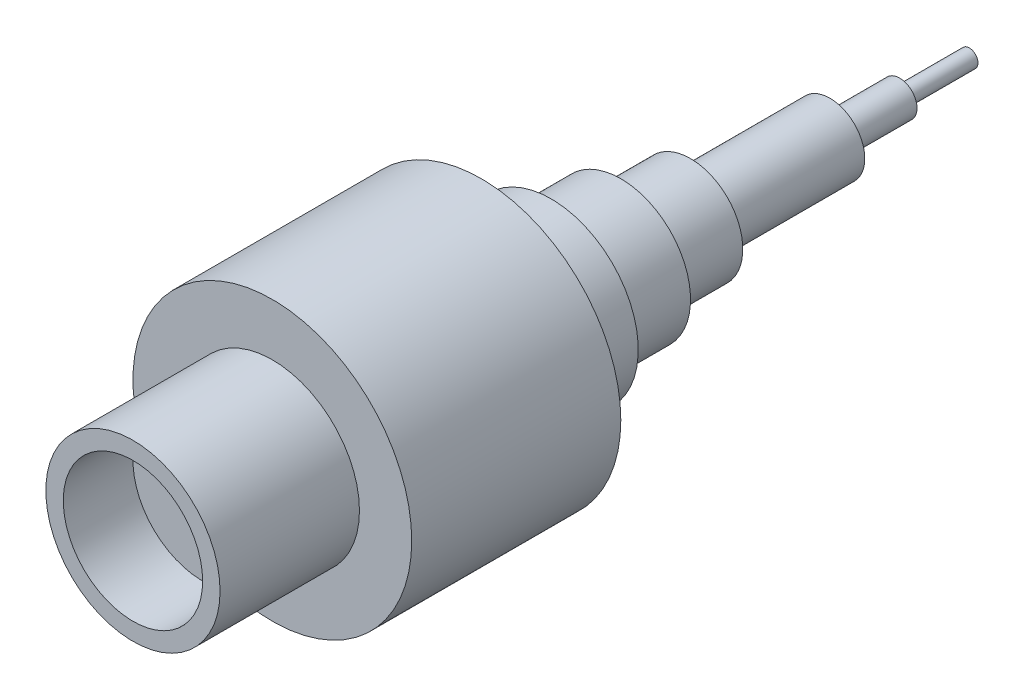
ISO-10303-21;
HEADER;
FILE_DESCRIPTION(('STEP AP214'),'2;1');
FILE_NAME('part.step','',(''),(''),'','','');
FILE_SCHEMA(('AUTOMOTIVE_DESIGN { 1 0 10303 214 1 1 1 1 }'));
ENDSEC;
DATA;
#1=APPLICATION_CONTEXT('core data for automotive mechanical design processes');
#2=APPLICATION_PROTOCOL_DEFINITION('international standard','automotive_design',2000,#1);
#3=PRODUCT_CONTEXT('',#1,'mechanical');
#4=PRODUCT('Part','Part','',(#3));
#5=PRODUCT_RELATED_PRODUCT_CATEGORY('part','',(#4));
#6=PRODUCT_DEFINITION_FORMATION('','',#4);
#7=PRODUCT_DEFINITION_CONTEXT('part definition',#1,'design');
#8=PRODUCT_DEFINITION('design','',#6,#7);
#9=PRODUCT_DEFINITION_SHAPE('','',#8);
#10=(LENGTH_UNIT() NAMED_UNIT(*) SI_UNIT(.MILLI.,.METRE.));
#11=(NAMED_UNIT(*) PLANE_ANGLE_UNIT() SI_UNIT($,.RADIAN.));
#12=(NAMED_UNIT(*) SI_UNIT($,.STERADIAN.) SOLID_ANGLE_UNIT());
#13=UNCERTAINTY_MEASURE_WITH_UNIT(LENGTH_MEASURE(1.E-05),#10,'distance_accuracy_value','');
#14=(GEOMETRIC_REPRESENTATION_CONTEXT(3) GLOBAL_UNCERTAINTY_ASSIGNED_CONTEXT((#13)) GLOBAL_UNIT_ASSIGNED_CONTEXT((#10,
#11,#12)) REPRESENTATION_CONTEXT('',''));
#15=CARTESIAN_POINT('',(0.,0.,0.));
#16=DIRECTION('',(0.,0.,1.));
#17=DIRECTION('',(1.,0.,0.));
#18=AXIS2_PLACEMENT_3D('',#15,#16,#17);
#19=CARTESIAN_POINT('',(0.,0.,60.));
#20=DIRECTION('',(0.,0.,-1.));
#21=DIRECTION('',(-1.,0.,0.));
#22=AXIS2_PLACEMENT_3D('',#19,#20,#21);
#23=CYLINDRICAL_SURFACE('',#22,40.);
#24=CARTESIAN_POINT('',(0.,0.,60.));
#25=DIRECTION('',(0.,0.,1.));
#26=DIRECTION('',(1.,0.,0.));
#27=AXIS2_PLACEMENT_3D('',#24,#25,#26);
#28=CIRCLE('',#27,40.);
#29=CARTESIAN_POINT('',(40.,0.,60.));
#30=VERTEX_POINT('',#29);
#31=EDGE_CURVE('E93',#30,#30,#28,.T.);
#32=ORIENTED_EDGE('',*,*,#31,.F.);
#33=EDGE_LOOP('',(#32));
#34=FACE_BOUND('',#33,.T.);
#35=CARTESIAN_POINT('',(0.,0.,0.));
#36=DIRECTION('',(0.,0.,1.));
#37=DIRECTION('',(1.,0.,0.));
#38=AXIS2_PLACEMENT_3D('',#35,#36,#37);
#39=CIRCLE('',#38,40.);
#40=CARTESIAN_POINT('',(40.,0.,0.));
#41=VERTEX_POINT('',#40);
#42=EDGE_CURVE('E37',#41,#41,#39,.T.);
#43=ORIENTED_EDGE('',*,*,#42,.T.);
#44=EDGE_LOOP('',(#43));
#45=FACE_BOUND('',#44,.T.);
#46=ADVANCED_FACE('F40',(#34,#45),#23,.T.);
#47=CARTESIAN_POINT('',(0.,0.,60.));
#48=DIRECTION('',(0.,0.,1.));
#49=DIRECTION('',(1.,0.,0.));
#50=AXIS2_PLACEMENT_3D('',#47,#48,#49);
#51=PLANE('',#50);
#52=CARTESIAN_POINT('',(0.,0.,60.));
#53=DIRECTION('',(0.,0.,1.));
#54=DIRECTION('',(1.,0.,0.));
#55=AXIS2_PLACEMENT_3D('',#52,#53,#54);
#56=CIRCLE('',#55,25.);
#57=CARTESIAN_POINT('',(25.,0.,60.));
#58=VERTEX_POINT('',#57);
#59=EDGE_CURVE('E81',#58,#58,#56,.T.);
#60=ORIENTED_EDGE('',*,*,#59,.F.);
#61=EDGE_LOOP('',(#60));
#62=FACE_BOUND('',#61,.T.);
#63=ORIENTED_EDGE('',*,*,#31,.T.);
#64=EDGE_LOOP('',(#63));
#65=FACE_BOUND('',#64,.T.);
#66=ADVANCED_FACE('F105',(#62,#65),#51,.T.);
#67=CARTESIAN_POINT('',(0.,0.,0.));
#68=DIRECTION('',(0.,0.,1.));
#69=DIRECTION('',(1.,0.,0.));
#70=AXIS2_PLACEMENT_3D('',#67,#68,#69);
#71=PLANE('',#70);
#72=CARTESIAN_POINT('',(0.,0.,0.));
#73=DIRECTION('',(0.,0.,-1.));
#74=DIRECTION('',(-1.,0.,0.));
#75=AXIS2_PLACEMENT_3D('',#72,#73,#74);
#76=CIRCLE('',#75,25.);
#77=CARTESIAN_POINT('',(-25.,0.,0.));
#78=VERTEX_POINT('',#77);
#79=EDGE_CURVE('E73',#78,#78,#76,.T.);
#80=ORIENTED_EDGE('',*,*,#79,.F.);
#81=EDGE_LOOP('',(#80));
#82=FACE_BOUND('',#81,.T.);
#83=ORIENTED_EDGE('',*,*,#42,.F.);
#84=EDGE_LOOP('',(#83));
#85=FACE_BOUND('',#84,.T.);
#86=ADVANCED_FACE('F97',(#82,#85),#71,.F.);
#87=CARTESIAN_POINT('',(0.,0.,100.));
#88=DIRECTION('',(0.,0.,-1.));
#89=DIRECTION('',(-1.,0.,0.));
#90=AXIS2_PLACEMENT_3D('',#87,#88,#89);
#91=CYLINDRICAL_SURFACE('',#90,25.);
#92=CARTESIAN_POINT('',(0.,0.,100.));
#93=DIRECTION('',(0.,0.,1.));
#94=DIRECTION('',(1.,0.,0.));
#95=AXIS2_PLACEMENT_3D('',#92,#93,#94);
#96=CIRCLE('',#95,25.);
#97=CARTESIAN_POINT('',(25.,0.,100.));
#98=VERTEX_POINT('',#97);
#99=EDGE_CURVE('E84',#98,#98,#96,.T.);
#100=ORIENTED_EDGE('',*,*,#99,.F.);
#101=EDGE_LOOP('',(#100));
#102=FACE_BOUND('',#101,.T.);
#103=ORIENTED_EDGE('',*,*,#59,.T.);
#104=EDGE_LOOP('',(#103));
#105=FACE_BOUND('',#104,.T.);
#106=ADVANCED_FACE('F101',(#102,#105),#91,.T.);
#107=CARTESIAN_POINT('',(0.,0.,100.));
#108=DIRECTION('',(0.,0.,1.));
#109=DIRECTION('',(1.,0.,0.));
#110=AXIS2_PLACEMENT_3D('',#107,#108,#109);
#111=PLANE('',#110);
#112=CARTESIAN_POINT('',(0.,0.,100.));
#113=DIRECTION('',(0.,0.,1.));
#114=DIRECTION('',(1.,0.,0.));
#115=AXIS2_PLACEMENT_3D('',#112,#113,#114);
#116=CIRCLE('',#115,20.);
#117=CARTESIAN_POINT('',(20.,0.,100.));
#118=VERTEX_POINT('',#117);
#119=EDGE_CURVE('E78',#118,#118,#116,.T.);
#120=ORIENTED_EDGE('',*,*,#119,.F.);
#121=EDGE_LOOP('',(#120));
#122=FACE_BOUND('',#121,.T.);
#123=ORIENTED_EDGE('',*,*,#99,.T.);
#124=EDGE_LOOP('',(#123));
#125=FACE_BOUND('',#124,.T.);
#126=ADVANCED_FACE('F108',(#122,#125),#111,.T.);
#127=CARTESIAN_POINT('',(0.,0.,80.));
#128=DIRECTION('',(0.,0.,1.));
#129=DIRECTION('',(1.,0.,0.));
#130=AXIS2_PLACEMENT_3D('',#127,#128,#129);
#131=CYLINDRICAL_SURFACE('',#130,20.);
#132=CARTESIAN_POINT('',(0.,0.,80.));
#133=DIRECTION('',(0.,0.,1.));
#134=DIRECTION('',(1.,0.,0.));
#135=AXIS2_PLACEMENT_3D('',#132,#133,#134);
#136=CIRCLE('',#135,20.);
#137=CARTESIAN_POINT('',(20.,0.,80.));
#138=VERTEX_POINT('',#137);
#139=EDGE_CURVE('E85',#138,#138,#136,.T.);
#140=ORIENTED_EDGE('',*,*,#139,.F.);
#141=EDGE_LOOP('',(#140));
#142=FACE_BOUND('',#141,.T.);
#143=ORIENTED_EDGE('',*,*,#119,.T.);
#144=EDGE_LOOP('',(#143));
#145=FACE_BOUND('',#144,.T.);
#146=ADVANCED_FACE('F140',(#142,#145),#131,.F.);
#147=CARTESIAN_POINT('',(0.,0.,80.));
#148=DIRECTION('',(0.,0.,1.));
#149=DIRECTION('',(1.,0.,0.));
#150=AXIS2_PLACEMENT_3D('',#147,#148,#149);
#151=PLANE('',#150);
#152=ORIENTED_EDGE('',*,*,#139,.T.);
#153=EDGE_LOOP('',(#152));
#154=FACE_BOUND('',#153,.T.);
#155=ADVANCED_FACE('F144',(#154),#151,.T.);
#156=CARTESIAN_POINT('',(0.,0.,-20.));
#157=DIRECTION('',(0.,0.,1.));
#158=DIRECTION('',(1.,0.,0.));
#159=AXIS2_PLACEMENT_3D('',#156,#157,#158);
#160=CYLINDRICAL_SURFACE('',#159,25.);
#161=CARTESIAN_POINT('',(0.,0.,-20.));
#162=DIRECTION('',(0.,0.,-1.));
#163=DIRECTION('',(-1.,0.,0.));
#164=AXIS2_PLACEMENT_3D('',#161,#162,#163);
#165=CIRCLE('',#164,25.);
#166=CARTESIAN_POINT('',(-25.,0.,-20.));
#167=VERTEX_POINT('',#166);
#168=EDGE_CURVE('E75',#167,#167,#165,.T.);
#169=ORIENTED_EDGE('',*,*,#168,.F.);
#170=EDGE_LOOP('',(#169));
#171=FACE_BOUND('',#170,.T.);
#172=ORIENTED_EDGE('',*,*,#79,.T.);
#173=EDGE_LOOP('',(#172));
#174=FACE_BOUND('',#173,.T.);
#175=ADVANCED_FACE('F153',(#171,#174),#160,.T.);
#176=CARTESIAN_POINT('',(0.,0.,-20.));
#177=DIRECTION('',(0.,0.,-1.));
#178=DIRECTION('',(-1.,0.,0.));
#179=AXIS2_PLACEMENT_3D('',#176,#177,#178);
#180=PLANE('',#179);
#181=CARTESIAN_POINT('',(0.,0.,-20.));
#182=DIRECTION('',(0.,0.,-1.));
#183=DIRECTION('',(-1.,0.,0.));
#184=AXIS2_PLACEMENT_3D('',#181,#182,#183);
#185=CIRCLE('',#184,20.);
#186=CARTESIAN_POINT('',(-20.,0.,-20.));
#187=VERTEX_POINT('',#186);
#188=EDGE_CURVE('E68',#187,#187,#185,.T.);
#189=ORIENTED_EDGE('',*,*,#188,.F.);
#190=EDGE_LOOP('',(#189));
#191=FACE_BOUND('',#190,.T.);
#192=ORIENTED_EDGE('',*,*,#168,.T.);
#193=EDGE_LOOP('',(#192));
#194=FACE_BOUND('',#193,.T.);
#195=ADVANCED_FACE('F164',(#191,#194),#180,.T.);
#196=CARTESIAN_POINT('',(0.,0.,-40.));
#197=DIRECTION('',(0.,0.,1.));
#198=DIRECTION('',(1.,0.,0.));
#199=AXIS2_PLACEMENT_3D('',#196,#197,#198);
#200=CYLINDRICAL_SURFACE('',#199,20.);
#201=CARTESIAN_POINT('',(0.,0.,-40.));
#202=DIRECTION('',(0.,0.,-1.));
#203=DIRECTION('',(-1.,0.,0.));
#204=AXIS2_PLACEMENT_3D('',#201,#202,#203);
#205=CIRCLE('',#204,20.);
#206=CARTESIAN_POINT('',(-20.,0.,-40.));
#207=VERTEX_POINT('',#206);
#208=EDGE_CURVE('E66',#207,#207,#205,.T.);
#209=ORIENTED_EDGE('',*,*,#208,.F.);
#210=EDGE_LOOP('',(#209));
#211=FACE_BOUND('',#210,.T.);
#212=ORIENTED_EDGE('',*,*,#188,.T.);
#213=EDGE_LOOP('',(#212));
#214=FACE_BOUND('',#213,.T.);
#215=ADVANCED_FACE('F171',(#211,#214),#200,.T.);
#216=CARTESIAN_POINT('',(0.,0.,-40.));
#217=DIRECTION('',(0.,0.,-1.));
#218=DIRECTION('',(-1.,0.,0.));
#219=AXIS2_PLACEMENT_3D('',#216,#217,#218);
#220=PLANE('',#219);
#221=CARTESIAN_POINT('',(0.,0.,-40.));
#222=DIRECTION('',(0.,0.,-1.));
#223=DIRECTION('',(-1.,0.,0.));
#224=AXIS2_PLACEMENT_3D('',#221,#222,#223);
#225=CIRCLE('',#224,15.);
#226=CARTESIAN_POINT('',(-15.,0.,-40.));
#227=VERTEX_POINT('',#226);
#228=EDGE_CURVE('E63',#227,#227,#225,.T.);
#229=ORIENTED_EDGE('',*,*,#228,.F.);
#230=EDGE_LOOP('',(#229));
#231=FACE_BOUND('',#230,.T.);
#232=ORIENTED_EDGE('',*,*,#208,.T.);
#233=EDGE_LOOP('',(#232));
#234=FACE_BOUND('',#233,.T.);
#235=ADVANCED_FACE('F183',(#231,#234),#220,.T.);
#236=CARTESIAN_POINT('',(0.,0.,-60.));
#237=DIRECTION('',(0.,0.,1.));
#238=DIRECTION('',(1.,0.,0.));
#239=AXIS2_PLACEMENT_3D('',#236,#237,#238);
#240=CYLINDRICAL_SURFACE('',#239,15.);
#241=CARTESIAN_POINT('',(0.,0.,-60.));
#242=DIRECTION('',(0.,0.,-1.));
#243=DIRECTION('',(-1.,0.,0.));
#244=AXIS2_PLACEMENT_3D('',#241,#242,#243);
#245=CIRCLE('',#244,15.);
#246=CARTESIAN_POINT('',(-15.,0.,-60.));
#247=VERTEX_POINT('',#246);
#248=EDGE_CURVE('E58',#247,#247,#245,.T.);
#249=ORIENTED_EDGE('',*,*,#248,.F.);
#250=EDGE_LOOP('',(#249));
#251=FACE_BOUND('',#250,.T.);
#252=ORIENTED_EDGE('',*,*,#228,.T.);
#253=EDGE_LOOP('',(#252));
#254=FACE_BOUND('',#253,.T.);
#255=ADVANCED_FACE('F194',(#251,#254),#240,.T.);
#256=CARTESIAN_POINT('',(0.,0.,-60.));
#257=DIRECTION('',(0.,0.,-1.));
#258=DIRECTION('',(-1.,0.,0.));
#259=AXIS2_PLACEMENT_3D('',#256,#257,#258);
#260=PLANE('',#259);
#261=CARTESIAN_POINT('',(0.,0.,-60.));
#262=DIRECTION('',(0.,0.,-1.));
#263=DIRECTION('',(-1.,0.,0.));
#264=AXIS2_PLACEMENT_3D('',#261,#262,#263);
#265=CIRCLE('',#264,10.);
#266=CARTESIAN_POINT('',(-10.,0.,-60.));
#267=VERTEX_POINT('',#266);
#268=EDGE_CURVE('E47',#267,#267,#265,.T.);
#269=ORIENTED_EDGE('',*,*,#268,.F.);
#270=EDGE_LOOP('',(#269));
#271=FACE_BOUND('',#270,.T.);
#272=ORIENTED_EDGE('',*,*,#248,.T.);
#273=EDGE_LOOP('',(#272));
#274=FACE_BOUND('',#273,.T.);
#275=ADVANCED_FACE('F202',(#271,#274),#260,.T.);
#276=CARTESIAN_POINT('',(0.,0.,-80.));
#277=DIRECTION('',(0.,0.,1.));
#278=DIRECTION('',(1.,0.,0.));
#279=AXIS2_PLACEMENT_3D('',#276,#277,#278);
#280=CYLINDRICAL_SURFACE('',#279,10.);
#281=ORIENTED_EDGE('',*,*,#268,.T.);
#282=EDGE_LOOP('',(#281));
#283=FACE_BOUND('',#282,.T.);
#284=CARTESIAN_POINT('',(0.,0.,-100.));
#285=DIRECTION('',(0.,0.,-1.));
#286=DIRECTION('',(-1.,0.,0.));
#287=AXIS2_PLACEMENT_3D('',#284,#285,#286);
#288=CIRCLE('',#287,10.);
#289=CARTESIAN_POINT('',(-10.,0.,-100.));
#290=VERTEX_POINT('',#289);
#291=EDGE_CURVE('E57',#290,#290,#288,.T.);
#292=ORIENTED_EDGE('',*,*,#291,.F.);
#293=EDGE_LOOP('',(#292));
#294=FACE_BOUND('',#293,.T.);
#295=ADVANCED_FACE('F214',(#283,#294),#280,.T.);
#296=CARTESIAN_POINT('',(0.,0.,-100.));
#297=DIRECTION('',(0.,0.,-1.));
#298=DIRECTION('',(-1.,0.,0.));
#299=AXIS2_PLACEMENT_3D('',#296,#297,#298);
#300=PLANE('',#299);
#301=CARTESIAN_POINT('',(0.,0.,-100.));
#302=DIRECTION('',(0.,0.,-1.));
#303=DIRECTION('',(-1.,0.,0.));
#304=AXIS2_PLACEMENT_3D('',#301,#302,#303);
#305=CIRCLE('',#304,5.);
#306=CARTESIAN_POINT('',(-5.,0.,-100.));
#307=VERTEX_POINT('',#306);
#308=EDGE_CURVE('E42',#307,#307,#305,.T.);
#309=ORIENTED_EDGE('',*,*,#308,.F.);
#310=EDGE_LOOP('',(#309));
#311=FACE_BOUND('',#310,.T.);
#312=ORIENTED_EDGE('',*,*,#291,.T.);
#313=EDGE_LOOP('',(#312));
#314=FACE_BOUND('',#313,.T.);
#315=ADVANCED_FACE('F223',(#311,#314),#300,.T.);
#316=CARTESIAN_POINT('',(0.,0.,-120.));
#317=DIRECTION('',(0.,0.,1.));
#318=DIRECTION('',(1.,0.,0.));
#319=AXIS2_PLACEMENT_3D('',#316,#317,#318);
#320=CYLINDRICAL_SURFACE('',#319,5.);
#321=CARTESIAN_POINT('',(0.,0.,-120.));
#322=DIRECTION('',(0.,0.,-1.));
#323=DIRECTION('',(-1.,0.,0.));
#324=AXIS2_PLACEMENT_3D('',#321,#322,#323);
#325=CIRCLE('',#324,5.);
#326=CARTESIAN_POINT('',(-5.,0.,-120.));
#327=VERTEX_POINT('',#326);
#328=EDGE_CURVE('E53',#327,#327,#325,.T.);
#329=ORIENTED_EDGE('',*,*,#328,.F.);
#330=EDGE_LOOP('',(#329));
#331=FACE_BOUND('',#330,.T.);
#332=ORIENTED_EDGE('',*,*,#308,.T.);
#333=EDGE_LOOP('',(#332));
#334=FACE_BOUND('',#333,.T.);
#335=ADVANCED_FACE('F236',(#331,#334),#320,.T.);
#336=CARTESIAN_POINT('',(0.,0.,-120.));
#337=DIRECTION('',(0.,0.,-1.));
#338=DIRECTION('',(-1.,0.,0.));
#339=AXIS2_PLACEMENT_3D('',#336,#337,#338);
#340=PLANE('',#339);
#341=CARTESIAN_POINT('',(0.,0.,-120.));
#342=DIRECTION('',(0.,0.,-1.));
#343=DIRECTION('',(-1.,0.,0.));
#344=AXIS2_PLACEMENT_3D('',#341,#342,#343);
#345=CIRCLE('',#344,2.5);
#346=CARTESIAN_POINT('',(-2.5,0.,-120.));
#347=VERTEX_POINT('',#346);
#348=EDGE_CURVE('E10',#347,#347,#345,.T.);
#349=ORIENTED_EDGE('',*,*,#348,.F.);
#350=EDGE_LOOP('',(#349));
#351=FACE_BOUND('',#350,.T.);
#352=ORIENTED_EDGE('',*,*,#328,.T.);
#353=EDGE_LOOP('',(#352));
#354=FACE_BOUND('',#353,.T.);
#355=ADVANCED_FACE('F247',(#351,#354),#340,.T.);
#356=CARTESIAN_POINT('',(0.,0.,-140.));
#357=DIRECTION('',(0.,0.,1.));
#358=DIRECTION('',(1.,0.,0.));
#359=AXIS2_PLACEMENT_3D('',#356,#357,#358);
#360=CYLINDRICAL_SURFACE('',#359,2.5);
#361=CARTESIAN_POINT('',(0.,0.,-140.));
#362=DIRECTION('',(0.,0.,-1.));
#363=DIRECTION('',(-1.,0.,0.));
#364=AXIS2_PLACEMENT_3D('',#361,#362,#363);
#365=CIRCLE('',#364,2.5);
#366=CARTESIAN_POINT('',(-2.5,0.,-140.));
#367=VERTEX_POINT('',#366);
#368=EDGE_CURVE('E52',#367,#367,#365,.T.);
#369=ORIENTED_EDGE('',*,*,#368,.F.);
#370=EDGE_LOOP('',(#369));
#371=FACE_BOUND('',#370,.T.);
#372=ORIENTED_EDGE('',*,*,#348,.T.);
#373=EDGE_LOOP('',(#372));
#374=FACE_BOUND('',#373,.T.);
#375=ADVANCED_FACE('F256',(#371,#374),#360,.T.);
#376=CARTESIAN_POINT('',(0.,0.,-140.));
#377=DIRECTION('',(0.,0.,-1.));
#378=DIRECTION('',(-1.,0.,0.));
#379=AXIS2_PLACEMENT_3D('',#376,#377,#378);
#380=PLANE('',#379);
#381=ORIENTED_EDGE('',*,*,#368,.T.);
#382=EDGE_LOOP('',(#381));
#383=FACE_BOUND('',#382,.T.);
#384=ADVANCED_FACE('F268',(#383),#380,.T.);
#385=CLOSED_SHELL('',(#46,#66,#86,#106,#126,#146,#155,#175,#195,#215,#235,#255,#275,#295,#315,
#335,#355,#375,#384));
#386=MANIFOLD_SOLID_BREP('B2',#385);
#387=ADVANCED_BREP_SHAPE_REPRESENTATION('',(#18,#386),#14);
#388=SHAPE_DEFINITION_REPRESENTATION(#9,#387);
ENDSEC;
END-ISO-10303-21;
